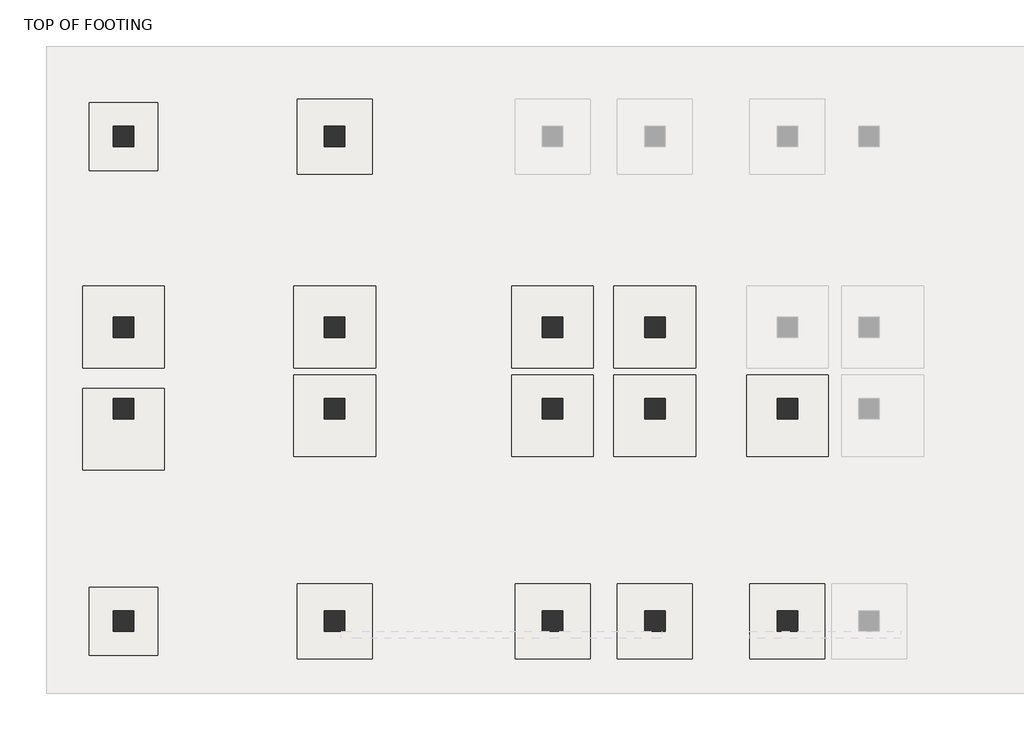
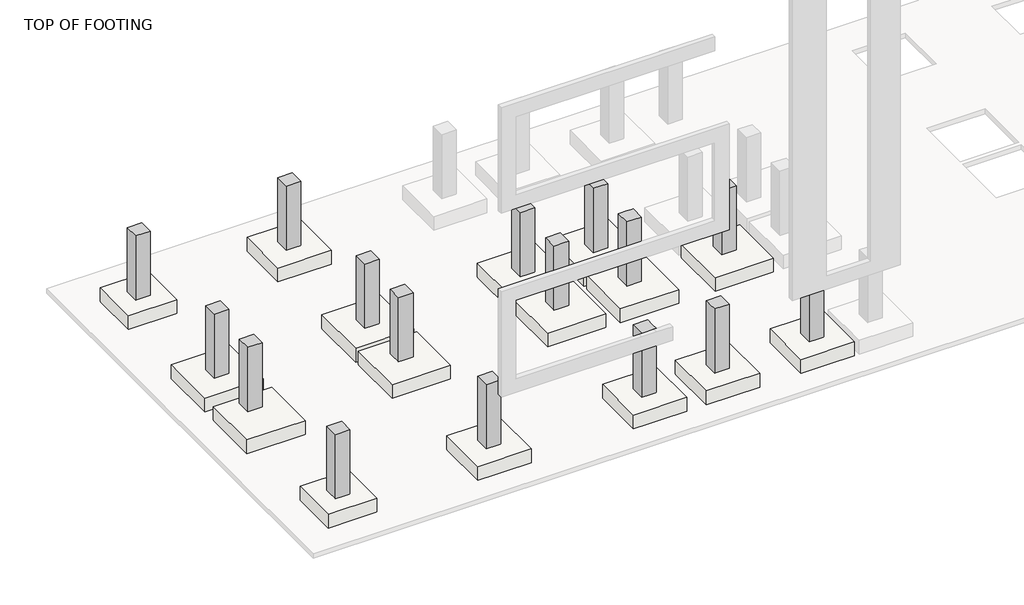
# One storey, part 1 of 2: 16 columns, 16 slabs.
"""IFC4 building model written with IfcOpenShell, lengths in millimetres."""

from ifc_helpers import new_model, si_unit, frame, origin, place, context, project, spatial, polyline, outline, extrude, faceted_brep, element, save

model = new_model("IFC4")

# Units and contexts
model_context = context("Model", 3, world=origin())
ifc_project = project(units=[si_unit("LENGTHUNIT", "METRE", prefix="MILLI")], contexts=[model_context])

# Site, building, storey
site = spatial("IfcSite", under=ifc_project)
building = spatial("IfcBuilding", under=site)
storey = spatial("IfcBuildingStorey", under=building, Name="TOP OF FOOTING", Elevation=-1828.8)

# Columns
placement = place(None, origin())
element("IfcColumn", 1, ObjectType="Concrete-Rectangular-Column : COLUMN 18\" X 18\"", at=placement, inside=storey, context=model_context, shape_type="SweptSolid", body=[
    extrude(outline(polyline([(-14916.7456086, 194.8205296), (-14916.7456086, -262.3794704), (-15373.9456086, -262.3794704), (-15373.9456086, 194.8205296), (-14916.7456086, 194.8205296)])), frame((0.0, 0.0, -1828.8), z_axis=(0.0, 0.0, 1.0), x_axis=(1.0, 0.0, 0.0)), (0.0, 0.0, 1.0), 2133.6),
])
element("IfcColumn", 2, ObjectType="Concrete-Rectangular-Column : COLUMN 18\" X 18\"", at=placement, inside=storey, context=model_context, shape_type="SweptSolid", body=[
    extrude(outline(polyline([(-10192.3456086, 194.8205296), (-10192.3456086, -262.3794704), (-10649.5456086, -262.3794704), (-10649.5456086, 194.8205296), (-10192.3456086, 194.8205296)])), frame((0.0, 0.0, -1828.8), z_axis=(0.0, 0.0, 1.0), x_axis=(1.0, 0.0, 0.0)), (0.0, 0.0, 1.0), 2133.6),
])
element("IfcColumn", 3, ObjectType="Concrete-Rectangular-Column : COLUMN 18\" X 18\"", at=placement, inside=storey, context=model_context, shape_type="SweptSolid", body=[
    extrude(outline(polyline([(-61.2083398, -10659.2679047), (-61.2083398, -11116.4679047), (-518.4083398, -11116.4679047), (-518.4083398, -10659.2679047), (-61.2083398, -10659.2679047)])), frame((0.0, 0.0, -1828.8), z_axis=(0.0, 0.0, 1.0), x_axis=(1.0, 0.0, 0.0)), (0.0, 0.0, 1.0), 2133.6),
])
element("IfcColumn", 4, ObjectType="Concrete-Rectangular-Column : COLUMN 18\" X 18\"", at=placement, inside=storey, context=model_context, shape_type="Brep", body=[
    faceted_brep([(-3029.5456086, -10659.2679047, -1828.8), (-3029.5456086, -11116.4679047, -1828.8), (-3486.7456086, -11116.4679047, -1828.8), (-3486.7456086, -10659.2679047, -1828.8), (-3029.5456086, -10659.2679047, 304.8), (-3029.5456086, -11116.4679047, 304.8), (-3486.7456086, -11116.4679047, 304.8), (-3486.7456086, -10887.8679047, 304.8), (-3486.7456086, -10659.2679047, 304.8), (-3486.7456086, -10659.2679047, 152.4)], [[[0, 1, 2, 3]], [[1, 0, 4, 5]], [[2, 1, 5, 6]], [[3, 2, 6, 7, 8, 9]], [[0, 3, 9, 8, 4]], [[5, 4, 8, 7, 6]]]),
])
element("IfcColumn", 5, ObjectType="Concrete-Rectangular-Column : COLUMN 18\" X 18\"", at=placement, inside=storey, context=model_context, shape_type="Brep", body=[
    faceted_brep([(-5315.5456086, -10659.2679047, -1828.8), (-5315.5456086, -11116.4679047, -1828.8), (-5772.7456086, -11116.4679047, -1828.8), (-5772.7456086, -10659.2679047, -1828.8), (-5315.5456086, -10659.2679047, 152.4), (-5315.5456086, -10659.2679047, 304.8), (-5315.5456086, -10887.8679047, 304.8), (-5315.5456086, -11116.4679047, 304.8), (-5772.7456086, -11116.4679047, 304.8), (-5772.7456086, -10659.2679047, 304.8), (-5417.1456086, -10659.2679047, 304.8)], [[[0, 1, 2, 3]], [[1, 0, 4, 5, 6, 7]], [[2, 1, 7, 8]], [[3, 2, 8, 9]], [[0, 3, 9, 10, 5, 4]], [[8, 7, 6, 5, 10, 9]]]),
])
element("IfcColumn", 6, ObjectType="Concrete-Rectangular-Column : COLUMN 18\" X 18\"", at=placement, inside=storey, context=model_context, shape_type="SweptSolid", body=[
    extrude(outline(polyline([(-10192.3456086, -10659.2679047), (-10192.3456086, -11116.4679047), (-10649.5456086, -11116.4679047), (-10649.5456086, -10659.2679047), (-10192.3456086, -10659.2679047)])), frame((0.0, 0.0, -1828.8), z_axis=(0.0, 0.0, 1.0), x_axis=(1.0, 0.0, 0.0)), (0.0, 0.0, 1.0), 2133.6),
])
element("IfcColumn", 7, ObjectType="Concrete-Rectangular-Column : COLUMN 18\" X 18\"", at=placement, inside=storey, context=model_context, shape_type="SweptSolid", body=[
    extrude(outline(polyline([(-14916.7456086, -10659.2679047), (-14916.7456086, -11116.4679047), (-15373.9456086, -11116.4679047), (-15373.9456086, -10659.2679047), (-14916.7456086, -10659.2679047)])), frame((0.0, 0.0, -1828.8), z_axis=(0.0, 0.0, 1.0), x_axis=(1.0, 0.0, 0.0)), (0.0, 0.0, 1.0), 2133.6),
])
element("IfcColumn", 8, ObjectType="Concrete-Rectangular-Column : COLUMN 18\" X 18\"", at=placement, inside=storey, context=model_context, shape_type="SweptSolid", body=[
    extrude(outline(polyline([(-14916.7456086, -5901.1794704), (-14916.7456086, -6358.3794704), (-15373.9456086, -6358.3794704), (-15373.9456086, -5901.1794704), (-14916.7456086, -5901.1794704)])), frame((0.0, 0.0, -1828.8), z_axis=(0.0, 0.0, 1.0), x_axis=(1.0, 0.0, 0.0)), (0.0, 0.0, 1.0), 2133.6),
])
element("IfcColumn", 9, ObjectType="Concrete-Rectangular-Column : COLUMN 18\" X 18\"", at=placement, inside=storey, context=model_context, shape_type="SweptSolid", body=[
    extrude(outline(polyline([(-14916.7456086, -4072.3794704), (-14916.7456086, -4529.5794704), (-15373.9456086, -4529.5794704), (-15373.9456086, -4072.3794704), (-14916.7456086, -4072.3794704)])), frame((0.0, 0.0, -1828.8), z_axis=(0.0, 0.0, 1.0), x_axis=(1.0, 0.0, 0.0)), (0.0, 0.0, 1.0), 2133.6),
])
element("IfcColumn", 10, ObjectType="Concrete-Rectangular-Column : COLUMN 18\" X 18\"", at=placement, inside=storey, context=model_context, shape_type="Brep", body=[
    faceted_brep([(-10192.3456086, -4072.3794704, -1828.8), (-10192.3456086, -4529.5794704, -1828.8), (-10649.5456086, -4529.5794704, -1828.8), (-10649.5456086, -4072.3794704, -1828.8), (-10192.3456086, -4072.3794704, 304.8), (-10192.3456086, -4529.5794704, 304.8), (-10192.3456086, -4529.5794704, 152.4), (-10649.5456086, -4529.5794704, 304.8), (-10649.5456086, -4529.5794704, 152.4), (-10649.5456086, -4072.3794704, 304.8)], [[[0, 1, 2, 3]], [[1, 0, 4, 5, 6]], [[2, 1, 6, 5, 7, 8]], [[3, 2, 8, 7, 9]], [[0, 3, 9, 4]], [[5, 4, 9, 7]]]),
])
element("IfcColumn", 11, ObjectType="Concrete-Rectangular-Column : COLUMN 18\" X 18\"", at=placement, inside=storey, context=model_context, shape_type="Brep", body=[
    faceted_brep([(-5315.5456086, -4072.3794704, -1828.8), (-5315.5456086, -4529.5794704, -1828.8), (-5772.7456086, -4529.5794704, -1828.8), (-5772.7456086, -4072.3794704, -1828.8), (-5315.5456086, -4072.3794704, 304.8), (-5315.5456086, -4529.5794704, 304.8), (-5315.5456086, -4529.5794704, 152.4), (-5772.7456086, -4529.5794704, 304.8), (-5772.7456086, -4529.5794704, 152.4), (-5772.7456086, -4072.3794704, 304.8)], [[[0, 1, 2, 3]], [[1, 0, 4, 5, 6]], [[2, 1, 6, 5, 7, 8]], [[3, 2, 8, 7, 9]], [[0, 3, 9, 4]], [[5, 4, 9, 7]]]),
])
element("IfcColumn", 12, ObjectType="Concrete-Rectangular-Column : COLUMN 18\" X 18\"", at=placement, inside=storey, context=model_context, shape_type="Brep", body=[
    faceted_brep([(-3029.5456086, -4072.3794704, -1828.8), (-3029.5456086, -4529.5794704, -1828.8), (-3486.7456086, -4529.5794704, -1828.8), (-3486.7456086, -4072.3794704, -1828.8), (-3029.5456086, -4072.3794704, 304.8), (-3029.5456086, -4529.5794704, 304.8), (-3029.5456086, -4529.5794704, 152.4), (-3486.7456086, -4529.5794704, 304.8), (-3486.7456086, -4529.5794704, 152.4), (-3486.7456086, -4072.3794704, 304.8)], [[[0, 1, 2, 3]], [[1, 0, 4, 5, 6]], [[2, 1, 6, 5, 7, 8]], [[3, 2, 8, 7, 9]], [[0, 3, 9, 4]], [[5, 4, 9, 7]]]),
])
element("IfcColumn", 13, ObjectType="Concrete-Rectangular-Column : COLUMN 18\" X 18\"", at=placement, inside=storey, context=model_context, shape_type="Brep", body=[
    faceted_brep([(-61.2083398, -5901.1794704, -1828.8), (-61.2083398, -6358.3794704, -1828.8), (-518.4083398, -6358.3794704, -1828.8), (-518.4083398, -5901.1794704, -1828.8), (-61.2083398, -5901.1794704, 152.4), (-61.2083398, -5901.1794704, 304.8), (-61.2083398, -6358.3794704, 304.8), (-518.4083398, -6358.3794704, 304.8), (-518.4083398, -5901.1794704, 304.8), (-518.4083398, -5901.1794704, 152.4)], [[[0, 1, 2, 3]], [[1, 0, 4, 5, 6]], [[2, 1, 6, 7]], [[3, 2, 7, 8, 9]], [[0, 3, 9, 8, 5, 4]], [[6, 5, 8, 7]]]),
])
element("IfcColumn", 14, ObjectType="Concrete-Rectangular-Column : COLUMN 18\" X 18\"", at=placement, inside=storey, context=model_context, shape_type="Brep", body=[
    faceted_brep([(-3029.5456086, -5901.1794704, -1828.8), (-3029.5456086, -6358.3794704, -1828.8), (-3486.7456086, -6358.3794704, -1828.8), (-3486.7456086, -5901.1794704, -1828.8), (-3029.5456086, -5901.1794704, 152.4), (-3029.5456086, -5901.1794704, 304.8), (-3029.5456086, -6358.3794704, 304.8), (-3486.7456086, -6358.3794704, 304.8), (-3486.7456086, -6358.3794704, 152.4), (-3486.7456086, -5901.1794704, 304.8), (-3486.7456086, -5901.1794704, 152.4), (-3232.7456086, -5901.1794704, 304.8), (-3105.7456086, -5901.1794704, 304.8)], [[[0, 1, 2, 3]], [[1, 0, 4, 5, 6]], [[2, 1, 6, 7, 8]], [[3, 2, 8, 7, 9, 10]], [[0, 3, 10, 9, 11, 12, 5, 4]], [[6, 5, 12, 11, 9, 7]]]),
])
element("IfcColumn", 15, ObjectType="Concrete-Rectangular-Column : COLUMN 18\" X 18\"", at=placement, inside=storey, context=model_context, shape_type="Brep", body=[
    faceted_brep([(-5315.5456086, -5901.1794704, -1828.8), (-5315.5456086, -6358.3794704, -1828.8), (-5772.7456086, -6358.3794704, -1828.8), (-5772.7456086, -5901.1794704, -1828.8), (-5315.5456086, -5901.1794704, 152.4), (-5315.5456086, -5901.1794704, 304.8), (-5315.5456086, -6358.3794704, 304.8), (-5315.5456086, -6358.3794704, 152.4), (-5417.1456086, -6358.3794704, 304.8), (-5772.7456086, -6358.3794704, 304.8), (-5772.7456086, -5901.1794704, 304.8), (-5772.7456086, -5901.1794704, 152.4)], [[[0, 1, 2, 3]], [[1, 0, 4, 5, 6, 7]], [[2, 1, 7, 6, 8, 9]], [[3, 2, 9, 10, 11]], [[0, 3, 11, 10, 5, 4]], [[6, 5, 10, 9, 8]]]),
])
element("IfcColumn", 16, ObjectType="Concrete-Rectangular-Column : COLUMN 18\" X 18\"", at=placement, inside=storey, context=model_context, shape_type="Brep", body=[
    faceted_brep([(-10192.3456086, -5901.1794704, -1828.8), (-10192.3456086, -6358.3794704, -1828.8), (-10649.5456086, -6358.3794704, -1828.8), (-10649.5456086, -5901.1794704, -1828.8), (-10192.3456086, -5901.1794704, 152.4), (-10192.3456086, -5901.1794704, 304.8), (-10192.3456086, -6358.3794704, 304.8), (-10649.5456086, -6358.3794704, 304.8), (-10649.5456086, -5901.1794704, 304.8), (-10649.5456086, -5901.1794704, 152.4)], [[[0, 1, 2, 3]], [[1, 0, 4, 5, 6]], [[2, 1, 6, 7]], [[3, 2, 7, 8, 9]], [[0, 3, 9, 8, 5, 4]], [[6, 5, 8, 7]]]),
])

# Slabs
element("IfcSlab", 17, ObjectType="Pile Cap-Rectangular : 5' 6\" X 5'6\" X 1'9\" EXTERIOR FOOTING", at=placement, inside=storey, context=model_context, shape_type="Brep", body=[
    faceted_brep([(-9582.7456086, 804.4205296, -1828.8), (-11259.1456086, 804.4205296, -1828.8), (-11259.1456086, -871.9794704, -1828.8), (-9582.7456086, -871.9794704, -1828.8), (-9582.7456086, 804.4205296, -2362.2), (-9582.7456086, -871.9794704, -2362.2), (-11259.1456086, -871.9794704, -2362.2), (-11259.1456086, 804.4205296, -2362.2), (-9582.7456086, 804.4205296, -2286.0), (-11259.1456086, 804.4205296, -2286.0), (-11259.1456086, -871.9794704, -2286.0), (-9582.7456086, -871.9794704, -2286.0)], [[[0, 1, 2, 3]], [[4, 5, 6, 7]], [[1, 0, 8, 4, 7, 9]], [[2, 1, 9, 7, 6, 10]], [[3, 2, 10, 6, 5, 11]], [[0, 3, 11, 5, 4, 8]]]),
])
element("IfcSlab", 18, ObjectType="Pile Cap-Rectangular : 5' 6\" X 5'6\" X 1'9\" EXTERIOR FOOTING", at=placement, inside=storey, context=model_context, shape_type="Brep", body=[
    faceted_brep([(-9582.7456086, -10049.6679047, -1828.8), (-11259.1456086, -10049.6679047, -1828.8), (-11259.1456086, -11726.0679047, -1828.8), (-9582.7456086, -11726.0679047, -1828.8), (-9582.7456086, -10049.6679047, -2362.2), (-9582.7456086, -11726.0679047, -2362.2), (-11259.1456086, -11726.0679047, -2362.2), (-11259.1456086, -10049.6679047, -2362.2), (-9582.7456086, -10049.6679047, -2286.0), (-11259.1456086, -10049.6679047, -2286.0), (-11259.1456086, -11726.0679047, -2286.0), (-9582.7456086, -11726.0679047, -2286.0)], [[[0, 1, 2, 3]], [[4, 5, 6, 7]], [[1, 0, 8, 4, 7, 9]], [[2, 1, 9, 7, 6, 10]], [[3, 2, 10, 6, 5, 11]], [[0, 3, 11, 5, 4, 8]]]),
])
element("IfcSlab", 19, ObjectType="Pile Cap-Rectangular : 5' 6\" X 5'6\" X 1'9\" EXTERIOR FOOTING", at=placement, inside=storey, context=model_context, shape_type="Brep", body=[
    faceted_brep([(-4705.9456086, -10049.6679047, -1828.8), (-6382.3456086, -10049.6679047, -1828.8), (-6382.3456086, -11726.0679047, -1828.8), (-4705.9456086, -11726.0679047, -1828.8), (-4705.9456086, -10049.6679047, -2362.2), (-4705.9456086, -11726.0679047, -2362.2), (-6382.3456086, -11726.0679047, -2362.2), (-6382.3456086, -10049.6679047, -2362.2), (-4705.9456086, -10049.6679047, -2286.0), (-6382.3456086, -10049.6679047, -2286.0), (-6382.3456086, -11726.0679047, -2286.0), (-4705.9456086, -11726.0679047, -2286.0)], [[[0, 1, 2, 3]], [[4, 5, 6, 7]], [[1, 0, 8, 4, 7, 9]], [[2, 1, 9, 7, 6, 10]], [[3, 2, 10, 6, 5, 11]], [[0, 3, 11, 5, 4, 8]]]),
])
element("IfcSlab", 20, ObjectType="Pile Cap-Rectangular : 5' 6\" X 5'6\" X 1'9\" EXTERIOR FOOTING", at=placement, inside=storey, context=model_context, shape_type="Brep", body=[
    faceted_brep([(-2419.9456086, -10049.6679047, -1828.8), (-4096.3456086, -10049.6679047, -1828.8), (-4096.3456086, -11726.0679047, -1828.8), (-2419.9456086, -11726.0679047, -1828.8), (-2419.9456086, -10049.6679047, -2362.2), (-2419.9456086, -11726.0679047, -2362.2), (-4096.3456086, -11726.0679047, -2362.2), (-4096.3456086, -10049.6679047, -2362.2), (-2419.9456086, -10049.6679047, -2286.0), (-4096.3456086, -10049.6679047, -2286.0), (-4096.3456086, -11726.0679047, -2286.0), (-2419.9456086, -11726.0679047, -2286.0)], [[[0, 1, 2, 3]], [[4, 5, 6, 7]], [[1, 0, 8, 4, 7, 9]], [[2, 1, 9, 7, 6, 10]], [[3, 2, 10, 6, 5, 11]], [[0, 3, 11, 5, 4, 8]]]),
])
element("IfcSlab", 21, ObjectType="Pile Cap-Rectangular : 5' 6\" X 5'6\" X 1'9\" EXTERIOR FOOTING", at=placement, inside=storey, context=model_context, shape_type="Brep", body=[
    faceted_brep([(548.3916602, -10049.6679047, -1828.8), (-1128.0083398, -10049.6679047, -1828.8), (-1128.0083398, -11726.0679047, -1828.8), (548.3916602, -11726.0679047, -1828.8), (548.3916602, -10049.6679047, -2362.2), (548.3916602, -11726.0679047, -2362.2), (-1128.0083398, -11726.0679047, -2362.2), (-1128.0083398, -10049.6679047, -2362.2), (548.3916602, -10049.6679047, -2286.0), (-1128.0083398, -10049.6679047, -2286.0), (-1128.0083398, -11726.0679047, -2286.0), (548.3916602, -11726.0679047, -2286.0)], [[[0, 1, 2, 3]], [[4, 5, 6, 7]], [[1, 0, 8, 4, 7, 9]], [[2, 1, 9, 7, 6, 10]], [[3, 2, 10, 6, 5, 11]], [[0, 3, 11, 5, 4, 8]]]),
])
element("IfcSlab", 22, ObjectType="Pile Cap-Rectangular : 5' X 5' X 1'9\" CORNER FOOTING", at=placement, inside=storey, context=model_context, shape_type="Brep", body=[
    faceted_brep([(-14383.3456086, -10125.8679047, -1828.8), (-15907.3456086, -10125.8679047, -1828.8), (-15907.3456086, -11649.8679047, -1828.8), (-14383.3456086, -11649.8679047, -1828.8), (-14383.3456086, -10125.8679047, -2362.2), (-14383.3456086, -11649.8679047, -2362.2), (-15907.3456086, -11649.8679047, -2362.2), (-15907.3456086, -10125.8679047, -2362.2), (-14383.3456086, -10125.8679047, -2286.0), (-15907.3456086, -10125.8679047, -2286.0), (-15907.3456086, -11649.8679047, -2286.0), (-14383.3456086, -11649.8679047, -2286.0)], [[[0, 1, 2, 3]], [[4, 5, 6, 7]], [[1, 0, 8, 4, 7, 9]], [[2, 1, 9, 7, 6, 10]], [[3, 2, 10, 6, 5, 11]], [[0, 3, 11, 5, 4, 8]]]),
])
element("IfcSlab", 23, ObjectType="Pile Cap-Rectangular : 5' X 5' X 1'9\" CORNER FOOTING", at=placement, inside=storey, context=model_context, shape_type="Brep", body=[
    faceted_brep([(-14383.3456086, 728.2205296, -1828.8), (-15907.3456086, 728.2205296, -1828.8), (-15907.3456086, -795.7794704, -1828.8), (-14383.3456086, -795.7794704, -1828.8), (-14383.3456086, 728.2205296, -2362.2), (-14383.3456086, -795.7794704, -2362.2), (-15907.3456086, -795.7794704, -2362.2), (-15907.3456086, 728.2205296, -2362.2), (-14383.3456086, 728.2205296, -2286.0), (-15907.3456086, 728.2205296, -2286.0), (-15907.3456086, -795.7794704, -2286.0), (-14383.3456086, -795.7794704, -2286.0)], [[[0, 1, 2, 3]], [[4, 5, 6, 7]], [[1, 0, 8, 4, 7, 9]], [[2, 1, 9, 7, 6, 10]], [[3, 2, 10, 6, 5, 11]], [[0, 3, 11, 5, 4, 8]]]),
])
element("IfcSlab", 24, ObjectType="Pile Cap-Rectangular : 6' X 6' X 2' FOOTING INTERIOR", at=placement, inside=storey, context=model_context, shape_type="Brep", body=[
    faceted_brep([(-14230.9456086, -3386.5794704, -1828.8), (-16059.7456086, -3386.5794704, -1828.8), (-16059.7456086, -5215.3794704, -1828.8), (-14230.9456086, -5215.3794704, -1828.8), (-14230.9456086, -3386.5794704, -2438.4), (-14230.9456086, -5215.3794704, -2438.4), (-16059.7456086, -5215.3794704, -2438.4), (-16059.7456086, -3386.5794704, -2438.4), (-14230.9456086, -3386.5794704, -2286.0), (-16059.7456086, -3386.5794704, -2286.0), (-16059.7456086, -5215.3794704, -2286.0), (-14230.9456086, -5215.3794704, -2286.0)], [[[0, 1, 2, 3]], [[4, 5, 6, 7]], [[1, 0, 8, 4, 7, 9]], [[2, 1, 9, 7, 6, 10]], [[3, 2, 10, 6, 5, 11]], [[0, 3, 11, 5, 4, 8]]]),
])
element("IfcSlab", 25, ObjectType="Pile Cap-Rectangular : 6' X 6' X 2' FOOTING INTERIOR", at=placement, inside=storey, context=model_context, shape_type="Brep", body=[
    faceted_brep([(-14230.9456086, -5672.5794704, -1828.8), (-16059.7456086, -5672.5794704, -1828.8), (-16059.7456086, -7501.3794704, -1828.8), (-14230.9456086, -7501.3794704, -1828.8), (-14230.9456086, -5672.5794704, -2438.4), (-14230.9456086, -7501.3794704, -2438.4), (-16059.7456086, -7501.3794704, -2438.4), (-16059.7456086, -5672.5794704, -2438.4), (-14230.9456086, -5672.5794704, -2286.0), (-16059.7456086, -5672.5794704, -2286.0), (-16059.7456086, -7501.3794704, -2286.0), (-14230.9456086, -7501.3794704, -2286.0)], [[[0, 1, 2, 3]], [[4, 5, 6, 7]], [[1, 0, 8, 4, 7, 9]], [[2, 1, 9, 7, 6, 10]], [[3, 2, 10, 6, 5, 11]], [[0, 3, 11, 5, 4, 8]]]),
])
element("IfcSlab", 26, ObjectType="Pile Cap-Rectangular : 6' X 6' X 2' FOOTING INTERIOR", at=placement, inside=storey, context=model_context, shape_type="Brep", body=[
    faceted_brep([(-9506.5456086, -3386.5794704, -1828.8), (-11335.3456086, -3386.5794704, -1828.8), (-11335.3456086, -5215.3794704, -1828.8), (-9506.5456086, -5215.3794704, -1828.8), (-9506.5456086, -3386.5794704, -2438.4), (-9506.5456086, -5215.3794704, -2438.4), (-11335.3456086, -5215.3794704, -2438.4), (-11335.3456086, -3386.5794704, -2438.4), (-9506.5456086, -3386.5794704, -2286.0), (-11335.3456086, -3386.5794704, -2286.0), (-11335.3456086, -5215.3794704, -2286.0), (-9506.5456086, -5215.3794704, -2286.0)], [[[0, 1, 2, 3]], [[4, 5, 6, 7]], [[1, 0, 8, 4, 7, 9]], [[2, 1, 9, 7, 6, 10]], [[3, 2, 10, 6, 5, 11]], [[0, 3, 11, 5, 4, 8]]]),
])
element("IfcSlab", 27, ObjectType="Pile Cap-Rectangular : 6' X 6' X 2' FOOTING INTERIOR", at=placement, inside=storey, context=model_context, shape_type="Brep", body=[
    faceted_brep([(-4629.7456086, -3386.5794704, -1828.8), (-6458.5456086, -3386.5794704, -1828.8), (-6458.5456086, -5215.3794704, -1828.8), (-4629.7456086, -5215.3794704, -1828.8), (-4629.7456086, -3386.5794704, -2438.4), (-4629.7456086, -5215.3794704, -2438.4), (-6458.5456086, -5215.3794704, -2438.4), (-6458.5456086, -3386.5794704, -2438.4), (-4629.7456086, -3386.5794704, -2286.0), (-6458.5456086, -3386.5794704, -2286.0), (-6458.5456086, -5215.3794704, -2286.0), (-4629.7456086, -5215.3794704, -2286.0)], [[[0, 1, 2, 3]], [[4, 5, 6, 7]], [[1, 0, 8, 4, 7, 9]], [[2, 1, 9, 7, 6, 10]], [[3, 2, 10, 6, 5, 11]], [[0, 3, 11, 5, 4, 8]]]),
])
element("IfcSlab", 28, ObjectType="Pile Cap-Rectangular : 6' X 6' X 2' FOOTING INTERIOR", at=placement, inside=storey, context=model_context, shape_type="Brep", body=[
    faceted_brep([(-2343.7456086, -3386.5794704, -1828.8), (-4172.5456086, -3386.5794704, -1828.8), (-4172.5456086, -5215.3794704, -1828.8), (-2343.7456086, -5215.3794704, -1828.8), (-2343.7456086, -3386.5794704, -2438.4), (-2343.7456086, -5215.3794704, -2438.4), (-4172.5456086, -5215.3794704, -2438.4), (-4172.5456086, -3386.5794704, -2438.4), (-2343.7456086, -3386.5794704, -2286.0), (-4172.5456086, -3386.5794704, -2286.0), (-4172.5456086, -5215.3794704, -2286.0), (-2343.7456086, -5215.3794704, -2286.0)], [[[0, 1, 2, 3]], [[4, 5, 6, 7]], [[1, 0, 8, 4, 7, 9]], [[2, 1, 9, 7, 6, 10]], [[3, 2, 10, 6, 5, 11]], [[0, 3, 11, 5, 4, 8]]]),
])
element("IfcSlab", 29, ObjectType="Pile Cap-Rectangular : 6' X 6' X 2' FOOTING INTERIOR", at=placement, inside=storey, context=model_context, shape_type="Brep", body=[
    faceted_brep([(624.5916602, -5367.7794704, -1828.8), (-1204.2083398, -5367.7794704, -1828.8), (-1204.2083398, -7196.5794704, -1828.8), (624.5916602, -7196.5794704, -1828.8), (624.5916602, -5367.7794704, -2438.4), (624.5916602, -7196.5794704, -2438.4), (-1204.2083398, -7196.5794704, -2438.4), (-1204.2083398, -5367.7794704, -2438.4), (624.5916602, -5367.7794704, -2286.0), (-1204.2083398, -5367.7794704, -2286.0), (-1204.2083398, -7196.5794704, -2286.0), (624.5916602, -7196.5794704, -2286.0)], [[[0, 1, 2, 3]], [[4, 5, 6, 7]], [[1, 0, 8, 4, 7, 9]], [[2, 1, 9, 7, 6, 10]], [[3, 2, 10, 6, 5, 11]], [[0, 3, 11, 5, 4, 8]]]),
])
element("IfcSlab", 30, ObjectType="Pile Cap-Rectangular : 6' X 6' X 2' FOOTING INTERIOR", at=placement, inside=storey, context=model_context, shape_type="Brep", body=[
    faceted_brep([(-2343.7456086, -5367.7794704, -1828.8), (-4172.5456086, -5367.7794704, -1828.8), (-4172.5456086, -7196.5794704, -1828.8), (-2343.7456086, -7196.5794704, -1828.8), (-2343.7456086, -5367.7794704, -2438.4), (-2343.7456086, -7196.5794704, -2438.4), (-4172.5456086, -7196.5794704, -2438.4), (-4172.5456086, -5367.7794704, -2438.4), (-2343.7456086, -5367.7794704, -2286.0), (-4172.5456086, -5367.7794704, -2286.0), (-4172.5456086, -7196.5794704, -2286.0), (-2343.7456086, -7196.5794704, -2286.0)], [[[0, 1, 2, 3]], [[4, 5, 6, 7]], [[1, 0, 8, 4, 7, 9]], [[2, 1, 9, 7, 6, 10]], [[3, 2, 10, 6, 5, 11]], [[0, 3, 11, 5, 4, 8]]]),
])
element("IfcSlab", 31, ObjectType="Pile Cap-Rectangular : 6' X 6' X 2' FOOTING INTERIOR", at=placement, inside=storey, context=model_context, shape_type="Brep", body=[
    faceted_brep([(-4629.7456086, -5367.7794704, -1828.8), (-6458.5456086, -5367.7794704, -1828.8), (-6458.5456086, -7196.5794704, -1828.8), (-4629.7456086, -7196.5794704, -1828.8), (-4629.7456086, -5367.7794704, -2438.4), (-4629.7456086, -7196.5794704, -2438.4), (-6458.5456086, -7196.5794704, -2438.4), (-6458.5456086, -5367.7794704, -2438.4), (-4629.7456086, -5367.7794704, -2286.0), (-6458.5456086, -5367.7794704, -2286.0), (-6458.5456086, -7196.5794704, -2286.0), (-4629.7456086, -7196.5794704, -2286.0)], [[[0, 1, 2, 3]], [[4, 5, 6, 7]], [[1, 0, 8, 4, 7, 9]], [[2, 1, 9, 7, 6, 10]], [[3, 2, 10, 6, 5, 11]], [[0, 3, 11, 5, 4, 8]]]),
])
element("IfcSlab", 32, ObjectType="Pile Cap-Rectangular : 6' X 6' X 2' FOOTING INTERIOR", at=placement, inside=storey, context=model_context, shape_type="Brep", body=[
    faceted_brep([(-9506.5456086, -5367.7794704, -1828.8), (-11335.3456086, -5367.7794704, -1828.8), (-11335.3456086, -7196.5794704, -1828.8), (-9506.5456086, -7196.5794704, -1828.8), (-9506.5456086, -5367.7794704, -2438.4), (-9506.5456086, -7196.5794704, -2438.4), (-11335.3456086, -7196.5794704, -2438.4), (-11335.3456086, -5367.7794704, -2438.4), (-9506.5456086, -5367.7794704, -2286.0), (-11335.3456086, -5367.7794704, -2286.0), (-11335.3456086, -7196.5794704, -2286.0), (-9506.5456086, -7196.5794704, -2286.0)], [[[0, 1, 2, 3]], [[4, 5, 6, 7]], [[1, 0, 8, 4, 7, 9]], [[2, 1, 9, 7, 6, 10]], [[3, 2, 10, 6, 5, 11]], [[0, 3, 11, 5, 4, 8]]]),
])

save(model, "model.ifc")

# Revit data of these elements
# Grids (mm)
#   "7": line (8545.813, 3363.463) -> (8545.813, -13331.65)
#   "1": line (-15145.346, 3363.463) -> (-15145.346, -13331.65)
#   "2": line (-10420.946, 3363.463) -> (-10420.946, -13331.65)
#   "3": line (-5544.146, 3363.463) -> (-5544.146, -13331.65)
#   "4": line (-3258.146, 3363.463) -> (-3258.146, -13331.65)
#   "6": line (1538.992, 3363.463) -> (1538.992, -13331.65)
#   "8": line (12813.013, 3363.463) -> (12813.013, -13331.65)
#   "C": line (15685.303, -6129.779) -> (-17668.837, -6129.779)
#   "D": line (15685.303, -10887.868) -> (-17668.837, -10887.868)
#   "E": line (-15145.346, 3363.463) -> (-15145.346, -13331.65)
#   "F": line (-10420.946, 3363.463) -> (-10420.946, -13331.65)
#   "G": line (-5544.146, 3363.463) -> (-5544.146, -13331.65)
#   "H": line (-3258.146, 3363.463) -> (-3258.146, -13331.65)
#   "I": line (-289.808, -13331.65) -> (-289.808, 3363.463)
#   "J": line (1538.992, 3363.463) -> (1538.992, -13331.65)
#   "K": line (8545.813, 3363.463) -> (8545.813, -13331.65)
#   "L": line (12813.013, 3363.463) -> (12813.013, -13331.65)
#   "M": line (15685.303, -33.779) -> (-17668.837, -33.779)
#   "N": line (15685.303, -4300.979) -> (-17668.837, -4300.979)
#   "O": line (15685.303, -6129.779) -> (-17668.837, -6129.779)
#   "P": line (15685.303, -10887.868) -> (-17668.837, -10887.868)
#   "Q": line (-15145.346, 3363.463) -> (-15145.346, -13331.65)
#   "R": line (-10420.946, 3363.463) -> (-10420.946, -13331.65)
#   "S": line (-5544.146, 3363.463) -> (-5544.146, -13331.65)
#   "T": line (-3258.146, 3363.463) -> (-3258.146, -13331.65)
#   "V": line (1538.992, 3363.463) -> (1538.992, -13331.65)
#   "W": line (8545.813, 3363.463) -> (8545.813, -13331.65)
#   "X": line (12813.013, 3363.463) -> (12813.013, -13331.65)
#   "Y": line (15685.303, -6129.779) -> (-17668.837, -6129.779)
#   "Z": line (15685.303, -10887.868) -> (-17668.837, -10887.868)
#   "AA": line (-15145.346, 3363.463) -> (-15145.346, -13331.65)
#   "BB": line (-10420.946, 3363.463) -> (-10420.946, -13331.65)
#   "CC": line (-5544.146, 3363.463) -> (-5544.146, -13331.65)
#   "DD": line (-3258.146, 3363.463) -> (-3258.146, -13331.65)
#   "EE": line (-289.808, -13331.65) -> (-289.808, 3363.463)
#   "FF": line (1538.992, 3363.463) -> (1538.992, -13331.65)
#   "GG": line (8545.813, 3363.463) -> (8545.813, -13331.65)
#   "HH": line (12813.013, 3363.463) -> (12813.013, -13331.65)
#   "II": line (15685.303, -33.779) -> (-17668.837, -33.779)
#   "JJ": line (15685.303, -4300.979) -> (-17668.837, -4300.979)
#   "KK": line (15685.303, -6129.779) -> (-17668.837, -6129.779)
#   "LL": line (15685.303, -10887.868) -> (-17668.837, -10887.868)
# Type "Concrete-Rectangular-Column : COLUMN 18\" X 18\""
#   Assembly Code = "B10"
#   b = 1' - 6"
#   h = 1' - 6"
#   Structural Material [instance default] = Concrete, Cast-in-Place gray
# Type "Pile Cap-Rectangular : 5' 6\" X 5'6\" X 1'9\" EXTERIOR FOOTING"
#   Assembly Code = "A1010100"
#   Width = 5' - 6"
#   Length = 5' - 6"
#   Foundation Thickness = 1' - 9"
#   Structural Material [instance default] = Concrete, Cast-in-Place gray
# Type "Pile Cap-Rectangular : 5' X 5' X 1'9\" CORNER FOOTING"
#   Assembly Code = "A1010100"
#   Width = 5' - 0"
#   Length = 5' - 0"
#   Foundation Thickness = 1' - 9"
#   Structural Material [instance default] = Concrete, Cast-in-Place gray
# Type "Pile Cap-Rectangular : 6' X 6' X 2' FOOTING INTERIOR"
#   Assembly Code = "A1010100"
#   Width = 6' - 0"
#   Length = 6' - 0"
#   Foundation Thickness = 2' - 0"
#   Structural Material [instance default] = Concrete, Cast-in-Place gray
# Elements 1, 2, 3, 4, 5, 6, 7, 8, 9, 10, 11, 12, 13, 14, 15, 16 (IfcColumn, "Concrete-Rectangular-Column : COLUMN 18\" X 18\"")
#   Structural Material = Concrete, Cast-in-Place gray
#   Phase Created = New Construction
#   Materials on its faces: "Concrete, Cast-in-Place gray"
# Elements 17, 18, 19, 20, 21 (IfcSlab, "Pile Cap-Rectangular : 5' 6\" X 5'6\" X 1'9\" EXTERIOR FOOTING")
#   Structural Material = Concrete, Cast-in-Place gray
#   Phase Created = New Construction
#   Materials on its faces: "Concrete, Cast-in-Place gray"
# Elements 22, 23 (IfcSlab, "Pile Cap-Rectangular : 5' X 5' X 1'9\" CORNER FOOTING")
#   Structural Material = Concrete, Cast-in-Place gray
#   Phase Created = New Construction
#   Materials on its faces: "Concrete, Cast-in-Place gray"
# Elements 24, 25, 26, 27, 28, 29, 30, 31, 32 (IfcSlab, "Pile Cap-Rectangular : 6' X 6' X 2' FOOTING INTERIOR")
#   Structural Material = Concrete, Cast-in-Place gray
#   Phase Created = New Construction
#   Materials on its faces: "Concrete, Cast-in-Place gray"
# Materials
#   "Concrete, Cast-in-Place gray": class "Concrete", colour RGB 192 192 192, transparency 0, Description = "Cast-in-place concrete", Cost = 0
